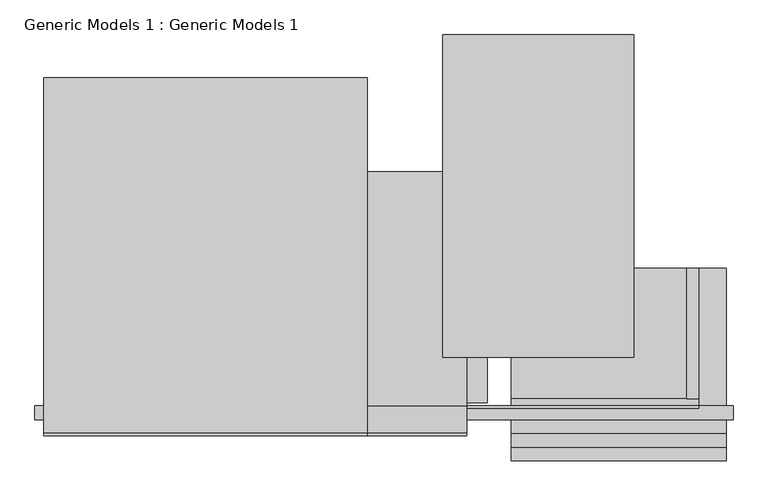
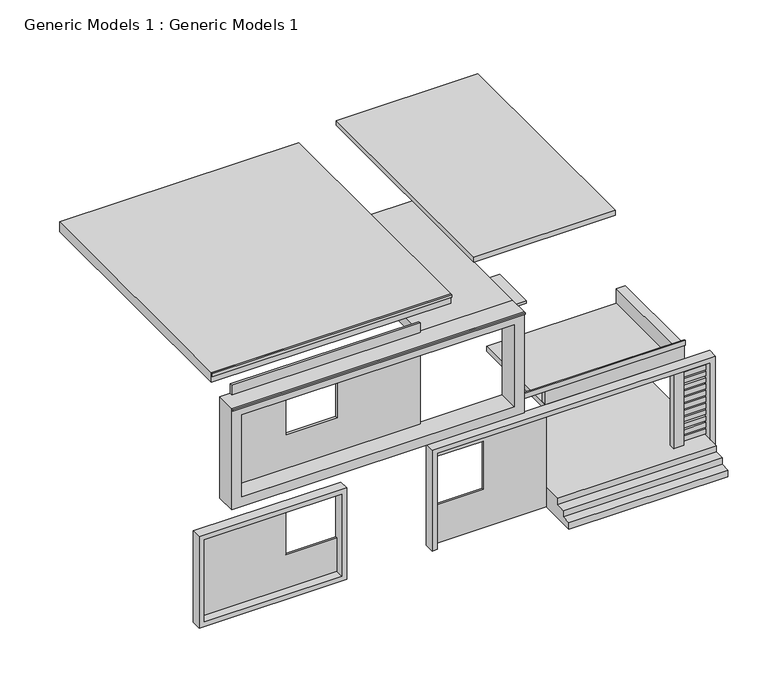
"""IFC4 building model written with IfcOpenShell, lengths in millimetres: proxy geometry, Generic Models 1 : Generic Models 1."""

from ifc_helpers import new_model, si_unit, frame, origin, origin_with_axes, place, context, project, spatial, polyline, outline, extrude, faceted_brep, source, transform, mapped, element, save


def generic_models_1_generic_models_1_b41e56dc(model_context):
    return source(origin(), model_context, "Body", "SolidModel", [
        extrude(outline(polyline([(-1808.3243879, -3803.7883122), (-8971.1243879, -3803.7883122), (-8971.1243879, -3752.9883122), (-1808.3243879, -3752.9883122), (-1808.3243879, -3803.7883122)])), frame((0.0, 0.0, 8115.3), z_axis=(0.0, 0.0, 1.0), x_axis=(1.0, 0.0, 0.0)), (0.0, 0.0, 1.0), 88.9),
        extrude(outline(polyline([(-8971.1243879, -3752.9883122), (-8971.1243879, 4121.0116878), (-1808.3243879, 4121.0116878), (-1808.3243879, -3752.9883122), (-8971.1243879, -3752.9883122)])), frame((0.0, 0.0, 7899.4), z_axis=(0.0, 0.0, 1.0), x_axis=(1.0, 0.0, 0.0)), (0.0, 0.0, 1.0), 304.8),
        extrude(outline(polyline([(-138.2743879, -2066.5910583), (-138.2743879, 5067.3185469), (4090.8256121, 5067.3185469), (4090.8256121, -2066.5910583), (-138.2743879, -2066.5910583)])), frame((0.0, 0.0, 7594.6), z_axis=(0.0, 0.0, 1.0), x_axis=(1.0, 0.0, 0.0)), (0.0, 0.0, 1.0), 152.4),
        extrude(outline(polyline([(5532.2756121, -3194.1883122), (393.8272859, -3194.1883122), (393.8272859, -3143.3883122), (5532.2756121, -3143.3883122), (5532.2756121, -3194.1883122)])), frame((0.0, 0.0, 3657.6), z_axis=(0.0, 0.0, 1.0), x_axis=(1.0, 0.0, 0.0)), (0.0, 0.0, 1.0), 152.4),
        extrude(outline(polyline([(-95.3883122, 609.6), (-95.3883122, 0.0), (-4362.5883122, 0.0), (-4362.5883122, 203.2), (-4057.7883122, 203.2), (-4057.7883122, 406.4), (-3752.9883122, 406.4), (-3752.9883122, 609.6), (-95.3883122, 609.6)])), frame((1379.3756121, 0.0, 0.0), z_axis=(1.0, 0.0, 0.0), x_axis=(0.0, 1.0, 0.0)), (0.0, 0.0, 1.0), 4762.5),
        extrude(outline(polyline([(5113.1756121, -3321.1883122), (5113.1756121, -3143.3883122), (5417.9756121, -3143.3883122), (5417.9756121, -3321.1883122), (5113.1756121, -3321.1883122)])), origin_with_axes(), (0.0, 0.0, 1.0), 3048.0),
        extrude(outline(polyline([(5417.9756121, -3219.5883122), (5417.9756121, -3143.3883122), (6141.8756121, -3143.3883122), (6141.8756121, -3219.5883122), (5417.9756121, -3219.5883122)])), frame((0.0, 0.0, 2895.850388), z_axis=(0.0, 0.0, 1.0), x_axis=(1.0, 0.0, 0.0)), (0.0, 0.0, 1.0), 152.149612),
        extrude(outline(polyline([(5417.9756121, -3219.5883122), (5417.9756121, -3143.3883122), (6141.8756121, -3143.3883122), (6141.8756121, -3219.5883122), (5417.9756121, -3219.5883122)])), frame((0.0, 0.0, 2692.650388), z_axis=(0.0, 0.0, 1.0), x_axis=(1.0, 0.0, 0.0)), (0.0, 0.0, 1.0), 152.4),
        extrude(outline(polyline([(5417.9756121, -3219.5883122), (5417.9756121, -3143.3883122), (6141.8756121, -3143.3883122), (6141.8756121, -3219.5883122), (5417.9756121, -3219.5883122)])), frame((0.0, 0.0, 2489.450388), z_axis=(0.0, 0.0, 1.0), x_axis=(1.0, 0.0, 0.0)), (0.0, 0.0, 1.0), 152.4),
        extrude(outline(polyline([(5417.9756121, -3219.5883122), (5417.9756121, -3143.3883122), (6141.8756121, -3143.3883122), (6141.8756121, -3219.5883122), (5417.9756121, -3219.5883122)])), frame((0.0, 0.0, 2286.250388), z_axis=(0.0, 0.0, 1.0), x_axis=(1.0, 0.0, 0.0)), (0.0, 0.0, 1.0), 152.4),
        extrude(outline(polyline([(5417.9756121, -3219.5883122), (5417.9756121, -3143.3883122), (6141.8756121, -3143.3883122), (6141.8756121, -3219.5883122), (5417.9756121, -3219.5883122)])), frame((0.0, 0.0, 2083.050388), z_axis=(0.0, 0.0, 1.0), x_axis=(1.0, 0.0, 0.0)), (0.0, 0.0, 1.0), 152.4),
        extrude(outline(polyline([(5417.9756121, -3219.5883122), (5417.9756121, -3143.3883122), (6141.8756121, -3143.3883122), (6141.8756121, -3219.5883122), (5417.9756121, -3219.5883122)])), frame((0.0, 0.0, 1879.850388), z_axis=(0.0, 0.0, 1.0), x_axis=(1.0, 0.0, 0.0)), (0.0, 0.0, 1.0), 152.4),
        extrude(outline(polyline([(5417.9756121, -3219.5883122), (5417.9756121, -3143.3883122), (6141.8756121, -3143.3883122), (6141.8756121, -3219.5883122), (5417.9756121, -3219.5883122)])), frame((0.0, 0.0, 1676.650388), z_axis=(0.0, 0.0, 1.0), x_axis=(1.0, 0.0, 0.0)), (0.0, 0.0, 1.0), 152.4),
        extrude(outline(polyline([(5417.9756121, -3219.5883122), (5417.9756121, -3143.3883122), (6141.8756121, -3143.3883122), (6141.8756121, -3219.5883122), (5417.9756121, -3219.5883122)])), frame((0.0, 0.0, 1473.450388), z_axis=(0.0, 0.0, 1.0), x_axis=(1.0, 0.0, 0.0)), (0.0, 0.0, 1.0), 152.4),
        extrude(outline(polyline([(5417.9756121, -3219.5883122), (5417.9756121, -3143.3883122), (6141.8756121, -3143.3883122), (6141.8756121, -3219.5883122), (5417.9756121, -3219.5883122)])), frame((0.0, 0.0, 1270.250388), z_axis=(0.0, 0.0, 1.0), x_axis=(1.0, 0.0, 0.0)), (0.0, 0.0, 1.0), 152.4),
        extrude(outline(polyline([(5417.9756121, -3219.5883122), (5417.9756121, -3143.3883122), (6141.8756121, -3143.3883122), (6141.8756121, -3219.5883122), (5417.9756121, -3219.5883122)])), frame((0.0, 0.0, 1067.050388), z_axis=(0.0, 0.0, 1.0), x_axis=(1.0, 0.0, 0.0)), (0.0, 0.0, 1.0), 152.4),
        extrude(outline(polyline([(5417.9756121, -3219.5883122), (5417.9756121, -3143.3883122), (6141.8756121, -3143.3883122), (6141.8756121, -3219.5883122), (5417.9756121, -3219.5883122)])), frame((0.0, 0.0, 863.850388), z_axis=(0.0, 0.0, 1.0), x_axis=(1.0, 0.0, 0.0)), (0.0, 0.0, 1.0), 152.4),
        extrude(outline(polyline([(5417.9756121, -3219.5883122), (5417.9756121, -3143.3883122), (6141.8756121, -3143.3883122), (6141.8756121, -3219.5883122), (5417.9756121, -3219.5883122)])), frame((0.0, 0.0, 660.650388), z_axis=(0.0, 0.0, 1.0), x_axis=(1.0, 0.0, 0.0)), (0.0, 0.0, 1.0), 152.4),
        faceted_brep([(6141.8756121, -3448.1883122, 3048.0), (6141.8756121, -3448.1883122, 0.0), (6294.2756121, -3448.1883122, 0.0), (6294.2756121, -3448.1883122, 3200.4), (-2189.3243879, -3448.1883122, 3200.4), (-2189.3243879, -3448.1883122, 0.0), (-2036.9243879, -3448.1883122, 0.0), (-2036.9243879, -3448.1883122, 3048.0), (6141.8756121, -3143.3883122, 3048.0), (-2036.9243879, -3143.3883122, 3048.0), (-2036.9243879, -3143.3883122, 0.0), (-2189.3243879, -3143.3883122, 0.0), (-2189.3243879, -3143.3883122, 3200.4), (6294.2756121, -3143.3883122, 3200.4), (6294.2756121, -3143.3883122, 0.0), (6141.8756121, -3143.3883122, 0.0), (6141.8756121, -3143.3883122, 203.450388), (6141.8756121, -3143.3883122, 254.250388), (6141.8756121, -3143.3883122, 406.650388), (6141.8756121, -3143.3883122, 457.450388), (6141.8756121, -3143.3883122, 609.850388), (6141.8756121, -3143.3883122, 660.650388), (6141.8756121, -3143.3883122, 813.050388), (6141.8756121, -3143.3883122, 863.850388), (6141.8756121, -3143.3883122, 1016.250388), (6141.8756121, -3143.3883122, 1067.050388), (6141.8756121, -3143.3883122, 1219.450388), (6141.8756121, -3143.3883122, 1270.250388), (6141.8756121, -3143.3883122, 1422.650388), (6141.8756121, -3143.3883122, 1473.450388), (6141.8756121, -3143.3883122, 1625.850388), (6141.8756121, -3143.3883122, 1676.650388), (6141.8756121, -3143.3883122, 1829.050388), (6141.8756121, -3143.3883122, 1879.850388), (6141.8756121, -3143.3883122, 2032.250388), (6141.8756121, -3143.3883122, 2083.050388), (6141.8756121, -3143.3883122, 2235.450388), (6141.8756121, -3143.3883122, 2286.250388), (6141.8756121, -3143.3883122, 2438.650388), (6141.8756121, -3143.3883122, 2489.450388), (6141.8756121, -3143.3883122, 2641.850388), (6141.8756121, -3143.3883122, 2692.650388), (6141.8756121, -3143.3883122, 2845.050388), (6141.8756121, -3143.3883122, 2895.850388), (5417.9756121, -3143.3883122, 3099.050388), (5417.9756121, -3143.3883122, 3048.250388), (6141.8756121, -3143.3883122, 3048.250388), (6141.8756121, -3143.3883122, 3099.050388), (5417.9756121, -3219.5883122, 3048.250388), (5417.9756121, -3219.5883122, 3099.050388), (6141.8756121, -3219.5883122, 3099.050388), (6141.8756121, -3219.5883122, 3048.250388)], [[[0, 1, 2, 3, 4, 5, 6, 7]], [[8, 9, 10, 11, 12, 13, 14, 15, 16, 17, 18, 19, 20, 21, 22, 23, 24, 25, 26, 27, 28, 29, 30, 31, 32, 33, 34, 35, 36, 37, 38, 39, 40, 41, 42, 43], [44, 45, 46, 47]], [[1, 0, 8, 43, 42, 41, 40, 39, 38, 37, 36, 35, 34, 33, 32, 31, 30, 29, 28, 27, 26, 25, 24, 23, 22, 21, 20, 19, 18, 17, 16, 15]], [[2, 1, 15, 14]], [[3, 2, 14, 13]], [[4, 3, 13, 12]], [[5, 4, 12, 11]], [[6, 5, 11, 10]], [[7, 6, 10, 9]], [[0, 7, 9, 8]], [[48, 49, 50, 51]], [[49, 48, 45, 44]], [[50, 49, 44, 47]], [[51, 50, 47, 46]], [[48, 51, 46, 45]]]),
        extrude(outline(polyline([(852.4853787, -1695.4314531), (852.4853787, -3072.9820671), (393.8272859, -3072.9820671), (393.8272859, -1695.4314531), (852.4853787, -1695.4314531)])), frame((0.0, 0.0, 6553.2), z_axis=(0.0, 0.0, 1.0), x_axis=(1.0, 0.0, 0.0)), (0.0, 0.0, 1.0), 81.3577548),
        extrude(outline(polyline([(393.8272859, -3803.7883122), (-8361.5243879, -3803.7883122), (-8361.5243879, -3752.9883122), (393.8272859, -3752.9883122), (393.8272859, -3803.7883122)])), frame((0.0, 0.0, 6807.2), z_axis=(0.0, 0.0, 1.0), x_axis=(1.0, 0.0, 0.0)), (0.0, 0.0, 1.0), 50.8),
        extrude(outline(polyline([(-2417.9243879, 2038.2116878), (393.8272859, 2038.2116878), (393.8272859, -3143.3883122), (-2417.9243879, -3143.3883122), (-2417.9243879, 2038.2116878)])), frame((0.0, 0.0, 6553.2), z_axis=(0.0, 0.0, 1.0), x_axis=(1.0, 0.0, 0.0)), (0.0, 0.0, 1.0), 304.8),
        extrude(outline(polyline([(7162.8, -2417.9243879), (7162.8, -8056.7243879), (3962.4, -8056.7243879), (3962.4, -2417.9243879), (7162.8, -2417.9243879)]), holes=[polyline([(6553.2, -4894.4243879), (5029.2, -4894.4243879), (5029.2, -6418.4243879), (6553.2, -6418.4243879), (6553.2, -4894.4243879)])]), frame((0.0, -3219.5883122, 0.0), z_axis=(0.0, 1.0, 0.0), x_axis=(0.0, 0.0, 1.0)), (0.0, 0.0, 1.0), 76.2),
        extrude(outline(polyline([(6858.0, 393.8272859), (6858.0, -8361.5243879), (3657.6, -8361.5243879), (3657.6, 393.8272859), (6858.0, 393.8272859)]), holes=[polyline([(6553.2, 89.0272859), (3962.4, 89.0272859), (3962.4, -8056.7243879), (6553.2, -8056.7243879), (6553.2, 89.0272859)])]), frame((0.0, -3752.9883122, 0.0), z_axis=(0.0, 1.0, 0.0), x_axis=(0.0, 0.0, 1.0)), (0.0, 0.0, 1.0), 609.6),
        extrude(outline(polyline([(1379.3756121, -95.3883122), (5532.2756121, -95.3883122), (5532.2756121, -3143.3883122), (1379.3756121, -3143.3883122), (1379.3756121, -95.3883122)])), frame((0.0, 0.0, 3048.0), z_axis=(0.0, 0.0, 1.0), x_axis=(1.0, 0.0, 0.0)), (0.0, 0.0, 1.0), 152.4),
        extrude(outline(polyline([(5265.5756121, -95.3883122), (5532.2756121, -95.3883122), (5532.2756121, -2990.9883122), (5265.5756121, -2990.9883122), (5265.5756121, -95.3883122)])), frame((0.0, 0.0, 3200.4), z_axis=(0.0, 0.0, 1.0), x_axis=(1.0, 0.0, 0.0)), (0.0, 0.0, 1.0), 457.2),
        extrude(outline(polyline([(5532.2756121, -2990.9883122), (5532.2756121, -3143.3883122), (1379.3756121, -3143.3883122), (1379.3756121, -2990.9883122), (5532.2756121, -2990.9883122)])), frame((0.0, 0.0, 3200.4), z_axis=(0.0, 0.0, 1.0), x_axis=(1.0, 0.0, 0.0)), (0.0, 0.0, 1.0), 457.2),
        extrude(outline(polyline([(3048.0, 1379.3756121), (3048.0, -2036.9243879), (2743.2, -2036.9243879), (2743.2, -512.9243879), (1219.2, -512.9243879), (1219.2, -2036.9243879), (0.0, -2036.9243879), (0.0, 1379.3756121), (3048.0, 1379.3756121)])), frame((0.0, -3194.1883122, 0.0), z_axis=(0.0, 1.0, 0.0), x_axis=(0.0, 0.0, 1.0)), (0.0, 0.0, 1.0), 50.8),
        extrude(outline(polyline([(1219.2, -6418.4243879), (2743.2, -6418.4243879), (2743.2, -9009.2243879), (0.0, -9009.2243879), (0.0, -4894.4243879), (1219.2, -4894.4243879), (1219.2, -6418.4243879)])), frame((0.0, -3194.1883122, 0.0), z_axis=(0.0, 1.0, 0.0), x_axis=(0.0, 0.0, 1.0)), (0.0, 0.0, 1.0), 50.8),
        extrude(outline(polyline([(2895.6, -9161.6243879), (0.0, -9161.6243879), (0.0, -4742.0243879), (2895.6, -4742.0243879), (2895.6, -9161.6243879)]), holes=[polyline([(2743.2, -9009.2243879), (2743.2, -4894.4243879), (152.4, -4894.4243879), (152.4, -9009.2243879), (2743.2, -9009.2243879)])]), frame((0.0, -3448.1883122, 0.0), z_axis=(0.0, 1.0, 0.0), x_axis=(0.0, 0.0, 1.0)), (0.0, 0.0, 1.0), 304.8),
    ])


if __name__ == "__main__":
    model = new_model("IFC4")
    model_context = context("Model", 3, world=origin())
    ifc_project = project(units=[si_unit("LENGTHUNIT", "METRE", prefix="MILLI")], contexts=[model_context])
    site = spatial("IfcSite", under=ifc_project)
    building = spatial("IfcBuilding", under=site)
    placement = place(None, origin())
    generic_models_1_generic_models_1_shape = generic_models_1_generic_models_1_b41e56dc(model_context)
    element("IfcBuildingElementProxy", 1, Name="Generic Models 1 : Generic Models 1", ObjectType="Generic Models 1 : Generic Models 1", at=placement, inside=building, context=model_context, shape_type="MappedRepresentation", body=[
        mapped(generic_models_1_generic_models_1_shape, transform((0.0, 0.0, 0.0), x_axis=(1.0, 0.0, 0.0), y_axis=(0.0, 1.0, 0.0), z_axis=(0.0, 0.0, 1.0))),
    ])
    save(model, "model.ifc")

# Revit data of these elements
# Element 1 (IfcBuildingElementProxy, "Generic Models 1 : Generic Models 1")
#   Materials on its faces: "Gypsum Wall Board", "Clad - White", "Wood Planks", "Ash colour"
# Materials
#   "Gypsum Wall Board": class "Generic", colour RGB 127 127 127, transparency 0, Description = "Gypsum Wall Board", Cost = 0
#   "Clad - White": class "Wood", colour RGB 242 242 238, transparency 0, Cost = 0
#   "Wood Planks": class "Wood", colour RGB 193 160 115, transparency 0, Description = "Physical material.", Cost = 0
#   "Ash colour": class "Generic", colour RGB 120 120 120, transparency 0, Cost = 0
